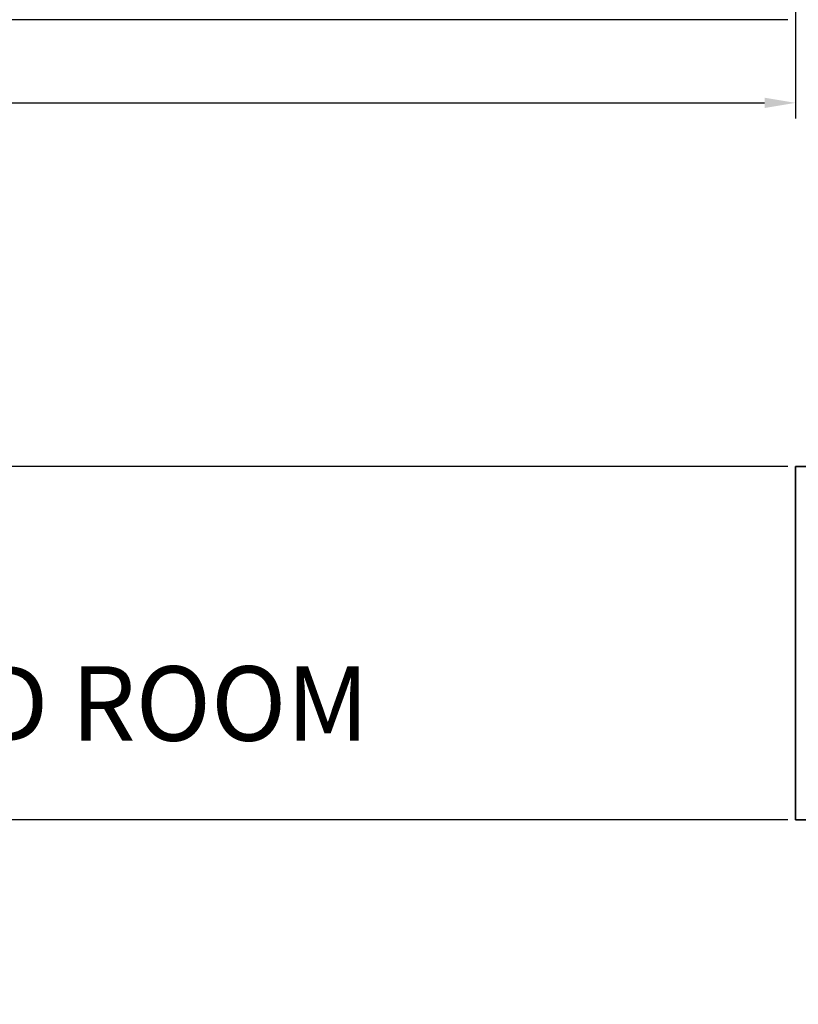
# Model space of a CAD drawing. Units: inches. Extents: x 2025 to 2528, y 1525 to 2336.
# Tile 14 of 18: x 2192 to 2255, y 2167 to 2246. Entities that reach past the tile are written whole.
import ezdxf

# ---------------------------------------------------------------- set-up
doc = ezdxf.new("R2010")
doc.units = ezdxf.units.IN
for name, color, linetype, lineweight in [('A-ANNO-DIMS', 2, 'Continuous', 18), ('A-AREA-IDEN', 7, 'Continuous', 25), ('A-FURN', 8, 'Continuous', 18), ('A-WALL', 7, 'Continuous', 35)]:
    doc.layers.add(name, color=color, linetype=linetype, lineweight=lineweight)
doc.styles.get("Standard").update_dxf_attribs({"font": 'arial.ttf'})
doc.dimstyles.new('Copy of ISO-25', dxfattribs={"dimtxt": 2.5, "dimasz": 2.5, "dimexe": 1.25, "dimexo": 0.625, "dimtad": 1, "dimdec": 1, "dimlunit": 4, "dimtxsty": 'Standard', "dimcen": 2.5, "dimadec": 0, "dimazin": 0, "dimtfac": 1, "dimtdec": 1, "dimtmove": 0, "dimatfit": 3, "dimfxl": 1, "dimarcsym": 0})

# ---------------------------------------------------------------- blocks, each defined once
blk = doc.blocks.new('*D6')
at = {"layer": 'A-ANNO-DIMS', "color": 0, "lineweight": -2, "transparency": 16777216}
for p, q in [((2075.013, 2282.787), (2075.013, 2237.927)), ((2255.013, 2282.787), (2255.013, 2237.927)), ((2077.513, 2239.177), (2252.513, 2239.177))]:
    blk.add_line(p, q, dxfattribs=at)
at = {"layer": 'A-ANNO-DIMS', "color": 0, "transparency": 16777216}
for points in [[(2077.513, 2239.594), (2077.513, 2238.761), (2075.013, 2239.177)], [(2252.513, 2239.594), (2252.513, 2238.761), (2255.013, 2239.177)]]:
    blk.add_solid(points, dxfattribs=at)
at = {"layer": 'Defpoints', "color": 0, "transparency": 16777216}
for p in [(2075.013, 2283.412), (2255.013, 2283.412), (2255.013, 2239.177)]:
    blk.add_point(p, dxfattribs=at)
at = {"layer": 'A-ANNO-DIMS', "color": 0, "transparency": 16777216, "insert": (2165.013, 2241.079), "char_height": 2.5, "attachment_point": 5}
blk.add_mtext("15'", dxfattribs=at)
blk = doc.blocks.new('A$C029D5C69')
for p, q in [((0.4164, 2.0693), (0.4164, 2.0066)), ((2.2315, 2.0693), (0.4164, 2.0693)), ((2.2315, 2.0066), (2.2315, 2.0693)), ((0, 1.606), (0, 2.0066)), ((0, 2.0066), (0.505, 2.0066)), ((0.0151, 1.6211), (0.0151, 1.9915)), ((0.0151, 1.9915), (0.4899, 1.9915)), ((0.4164, 2.0066), (2.2315, 2.0066)), ((0.4899, 1.9915), (0.4899, 1.6211)), ((0.505, 2.0066), (0.505, 1.606)), ((0.5252, 0.0351), (0.5252, 2.0066)), ((0.5403, 0.0502), (0.5403, 2.0066)), ((0.5706, 0.0805), (0.5706, 2.0066)), ((0.6869, 1.966), (0.6666, 2.0066)), ((0.7072, 2.0066), (0.6869, 1.966)), ((1.0902, 1.966), (1.0699, 2.0066)), ((1.1106, 2.0066), (1.0902, 1.966)), ((2.1114, 2.0087), (2.1114, 0.0351)), ((2.6479, 2.0066), (2.1429, 2.0066)), ((2.1429, 2.0066), (2.1429, 1.606)), ((2.6328, 1.9915), (2.158, 1.9915)), ((2.158, 1.9915), (2.158, 1.6211)), ((2.6328, 1.6211), (2.6328, 1.9915)), ((2.6479, 1.606), (2.6479, 2.0066)), ((0.6869, 1.9425), (0.6869, 1.966)), ((0.6869, 1.9425), (0.6869, 1.966)), ((1.0902, 1.9425), (1.0902, 1.966)), ((1.0902, 1.9425), (1.0902, 1.966)), ((1.8954, 1.9865), (1.3081, 1.9865)), ((1.8954, 1.9713), (1.3339, 1.9713)), ((1.3849, 1.9713), (1.3656, 1.952)), ((1.3945, 1.9713), (1.3714, 1.9483)), ((1.4249, 1.945), (1.3986, 1.9713)), ((1.4288, 1.9507), (1.4081, 1.9713)), ((1.487, 1.9713), (1.4664, 1.9507)), ((1.4966, 1.9713), (1.4703, 1.945)), ((1.527, 1.945), (1.5007, 1.9713)), ((1.5309, 1.9507), (1.5102, 1.9713)), ((1.5891, 1.9713), (1.5685, 1.9507)), ((1.5987, 1.9713), (1.5724, 1.945)), ((1.6291, 1.945), (1.6028, 1.9713)), ((1.633, 1.9507), (1.6123, 1.9713)), ((1.6912, 1.9713), (1.6706, 1.9507)), ((1.7008, 1.9713), (1.6745, 1.945)), ((1.7312, 1.945), (1.7049, 1.9713)), ((1.7351, 1.9507), (1.7144, 1.9713)), ((1.7933, 1.9713), (1.7727, 1.9507)), ((1.8029, 1.9713), (1.7766, 1.945)), ((1.8333, 1.945), (1.807, 1.9713)), ((1.8372, 1.9507), (1.8165, 1.9713)), ((1.8954, 1.9713), (1.8748, 1.9507)), ((1.9043, 1.9707), (1.8787, 1.945)), ((1.9354, 1.945), (1.9114, 1.969)), ((0.2689, 1.9609), (0.2689, 1.6764)), ((0.6634, 1.9425), (0.621, 1.9213)), ((0.6634, 1.9425), (0.621, 1.9213)), ((0.6869, 1.9425), (0.6634, 1.9425)), ((0.6869, 1.9425), (0.7104, 1.9425)), ((0.7528, 1.9213), (0.7104, 1.9425)), ((0.7528, 1.9213), (0.7104, 1.9425)), ((1.0668, 1.9425), (1.0244, 1.9213)), ((1.0668, 1.9425), (1.0244, 1.9213)), ((1.0902, 1.9425), (1.0668, 1.9425)), ((1.0902, 1.9425), (1.1137, 1.9425)), ((1.1561, 1.9213), (1.1137, 1.9425)), ((1.1561, 1.9213), (1.1137, 1.9425)), ((1.4249, 1.945), (1.4059, 1.926)), ((1.4288, 1.9394), (1.4116, 1.9222)), ((1.4476, 1.9507), (1.4288, 1.9507)), ((1.4288, 1.9393), (1.4476, 1.9393)), ((1.4476, 1.9507), (1.4664, 1.9507)), ((1.4664, 1.9393), (1.4476, 1.9393)), ((1.493, 1.9128), (1.4664, 1.9394)), ((1.4986, 1.9167), (1.4703, 1.945)), ((1.527, 1.945), (1.4986, 1.9167)), ((1.5309, 1.9394), (1.5043, 1.9128)), ((1.5497, 1.9507), (1.5309, 1.9507)), ((1.5309, 1.9393), (1.5497, 1.9393)), ((1.5497, 1.9507), (1.5685, 1.9507)), ((1.5685, 1.9393), (1.5497, 1.9393)), ((1.595, 1.9128), (1.5685, 1.9394)), ((1.6007, 1.9167), (1.5724, 1.945)), ((1.6291, 1.945), (1.6007, 1.9167)), ((1.633, 1.9394), (1.6064, 1.9128)), ((1.6518, 1.9507), (1.633, 1.9507)), ((1.633, 1.9393), (1.6518, 1.9393)), ((1.6518, 1.9507), (1.6706, 1.9507)), ((1.6706, 1.9393), (1.6518, 1.9393)), ((1.6971, 1.9128), (1.6706, 1.9394)), ((1.7028, 1.9167), (1.6745, 1.945)), ((1.7312, 1.945), (1.7028, 1.9167)), ((1.7351, 1.9394), (1.7085, 1.9128)), ((1.7539, 1.9507), (1.7351, 1.9507)), ((1.7351, 1.9393), (1.7539, 1.9393)), ((1.7539, 1.9507), (1.7727, 1.9507)), ((1.7727, 1.9393), (1.7539, 1.9393)), ((1.7992, 1.9128), (1.7727, 1.9394)), ((1.8049, 1.9167), (1.7766, 1.945)), ((1.8333, 1.945), (1.8049, 1.9167)), ((1.8372, 1.9394), (1.8106, 1.9128)), ((1.856, 1.9507), (1.8372, 1.9507)), ((1.8372, 1.9393), (1.856, 1.9393)), ((1.856, 1.9507), (1.8748, 1.9507)), ((1.8748, 1.9393), (1.856, 1.9393)), ((1.9013, 1.9128), (1.8748, 1.9394)), ((1.907, 1.9167), (1.8787, 1.945)), ((1.9354, 1.945), (1.907, 1.9167)), ((1.9393, 1.9394), (1.9127, 1.9128)), ((1.9393, 1.9393), (1.9404, 1.9393)), ((2.379, 1.9609), (2.379, 1.6764)), ((0.621, 1.9213), (0.5955, 1.8958)), ((0.7783, 1.8958), (0.7528, 1.9213)), ((1.0243, 1.9213), (0.9988, 1.8958)), ((1.1816, 1.8958), (1.1561, 1.9213)), ((1.9414, 1.688), (1.9414, 1.931)), ((1.9565, 1.688), (1.9565, 1.931)), ((0.5955, 1.8958), (0.5743, 1.8534)), ((0.7995, 1.8534), (0.7783, 1.8958)), ((0.9989, 1.8958), (0.9777, 1.8534)), ((1.2028, 1.8534), (1.1816, 1.8958)), ((1.493, 1.8752), (1.493, 1.9128)), ((1.5043, 1.8752), (1.5043, 1.9128)), ((1.595, 1.8752), (1.595, 1.9128)), ((1.6064, 1.8752), (1.6064, 1.9128)), ((1.6971, 1.8752), (1.6971, 1.9128)), ((1.7085, 1.8752), (1.7085, 1.9128)), ((1.7992, 1.8752), (1.7992, 1.9128)), ((1.8106, 1.8752), (1.8106, 1.9128)), ((1.9013, 1.8752), (1.9013, 1.9128)), ((1.9127, 1.8752), (1.9127, 1.9128)), ((1.493, 1.8752), (1.4867, 1.869)), ((1.4986, 1.8713), (1.4922, 1.8648)), ((1.527, 1.8429), (1.4986, 1.8713)), ((1.5309, 1.8486), (1.5043, 1.8752)), ((1.595, 1.8752), (1.5685, 1.8486)), ((1.6007, 1.8713), (1.5724, 1.8429)), ((1.6291, 1.8429), (1.6007, 1.8713)), ((1.633, 1.8486), (1.6064, 1.8752)), ((1.6971, 1.8752), (1.6706, 1.8486)), ((1.7028, 1.8713), (1.6745, 1.8429)), ((1.7312, 1.8429), (1.7028, 1.8713)), ((1.7351, 1.8486), (1.7085, 1.8752)), ((1.7992, 1.8752), (1.7727, 1.8486)), ((1.8049, 1.8713), (1.7766, 1.8429)), ((1.8333, 1.8429), (1.8049, 1.8713)), ((1.8372, 1.8486), (1.8106, 1.8752)), ((1.9013, 1.8752), (1.8748, 1.8486)), ((1.907, 1.8713), (1.8787, 1.8429)), ((1.9354, 1.8429), (1.907, 1.8713)), ((1.9393, 1.8486), (1.9127, 1.8752)), ((0.5743, 1.8534), (0.5706, 1.8515)), ((0.5743, 1.8534), (0.5706, 1.8515)), ((0.8419, 1.8322), (0.7995, 1.8534)), ((0.8419, 1.8322), (0.7995, 1.8534)), ((0.9777, 1.8534), (0.9353, 1.8322)), ((0.9777, 1.8534), (0.9353, 1.8322)), ((1.2452, 1.8322), (1.2028, 1.8534)), ((1.2452, 1.8322), (1.2028, 1.8534)), ((1.5497, 1.8486), (1.5309, 1.8486)), ((1.5497, 1.8486), (1.5685, 1.8486)), ((1.6518, 1.8486), (1.633, 1.8486)), ((1.6518, 1.8486), (1.6706, 1.8486)), ((1.7539, 1.8486), (1.7351, 1.8486)), ((1.7539, 1.8486), (1.7727, 1.8486)), ((1.856, 1.8486), (1.8372, 1.8486)), ((1.856, 1.8486), (1.8748, 1.8486)), ((1.9414, 1.8486), (1.9393, 1.8486)), ((0.8674, 1.8067), (0.8419, 1.8322)), ((0.9352, 1.8322), (0.9097, 1.8067)), ((1.2707, 1.8067), (1.2452, 1.8322)), ((1.527, 1.8429), (1.5242, 1.8401)), ((1.5309, 1.8373), (1.5295, 1.8359)), ((1.5309, 1.8373), (1.5497, 1.8373)), ((1.5685, 1.8373), (1.5497, 1.8373)), ((1.595, 1.8107), (1.5685, 1.8373)), ((1.6007, 1.8146), (1.5724, 1.8429)), ((1.6291, 1.8429), (1.6007, 1.8146)), ((1.633, 1.8373), (1.6064, 1.8107)), ((1.633, 1.8373), (1.6518, 1.8373)), ((1.6706, 1.8373), (1.6518, 1.8373)), ((1.6971, 1.8107), (1.6706, 1.8373)), ((1.7028, 1.8146), (1.6745, 1.8429)), ((1.7312, 1.8429), (1.7028, 1.8146)), ((1.7351, 1.8373), (1.7085, 1.8107)), ((1.7351, 1.8373), (1.7539, 1.8373)), ((1.7727, 1.8373), (1.7539, 1.8373)), ((1.7992, 1.8107), (1.7727, 1.8373)), ((1.8049, 1.8146), (1.7766, 1.8429)), ((1.8333, 1.8429), (1.8049, 1.8146)), ((1.8372, 1.8373), (1.8106, 1.8107)), ((1.8372, 1.8373), (1.856, 1.8373)), ((1.8748, 1.8373), (1.856, 1.8373)), ((1.9013, 1.8107), (1.8748, 1.8373)), ((1.907, 1.8146), (1.8787, 1.8429)), ((1.9354, 1.8429), (1.907, 1.8146)), ((1.9393, 1.8373), (1.9127, 1.8107)), ((1.9393, 1.8373), (1.9414, 1.8373)), ((0.1267, 1.8186), (0.4111, 1.8186)), ((0.8886, 1.7643), (0.8674, 1.8067)), ((0.9098, 1.8067), (0.8886, 1.7643)), ((1.2919, 1.7643), (1.2707, 1.8067)), ((1.595, 1.7806), (1.595, 1.8107)), ((1.6064, 1.7731), (1.6064, 1.8107)), ((1.6971, 1.7731), (1.6971, 1.8107)), ((1.7085, 1.7731), (1.7085, 1.8107)), ((1.7992, 1.7731), (1.7992, 1.8107)), ((1.8106, 1.7731), (1.8106, 1.8107)), ((1.9013, 1.7731), (1.9013, 1.8107)), ((1.9127, 1.7731), (1.9127, 1.8107)), ((2.2367, 1.8186), (2.5212, 1.8186)), ((1.2981, 1.7768), (1.2919, 1.7643)), ((1.633, 1.7465), (1.6064, 1.7731)), ((1.6971, 1.7731), (1.6706, 1.7465)), ((1.7351, 1.7465), (1.7085, 1.7731)), ((1.7992, 1.7731), (1.7727, 1.7465)), ((1.8372, 1.7465), (1.8106, 1.7731)), ((1.9013, 1.7731), (1.8748, 1.7465)), ((1.9393, 1.7465), (1.9127, 1.7731)), ((0.8886, 1.7408), (0.8886, 1.7643)), ((1.2919, 1.7519), (1.2919, 1.7643)), ((1.7028, 1.7692), (1.6745, 1.7408)), ((1.7312, 1.7408), (1.7028, 1.7692)), ((1.8049, 1.7692), (1.7766, 1.7408)), ((1.8333, 1.7408), (1.8049, 1.7692)), ((1.907, 1.7692), (1.8787, 1.7408)), ((1.9354, 1.7408), (1.907, 1.7692)), ((0.8651, 1.7408), (0.8227, 1.7196)), ((0.8651, 1.7408), (0.8227, 1.7196)), ((0.912, 1.7408), (0.8651, 1.7408)), ((0.9544, 1.7196), (0.912, 1.7408)), ((0.9544, 1.7196), (0.912, 1.7408)), ((1.2684, 1.7408), (1.226, 1.7196)), ((1.2684, 1.7408), (1.226, 1.7196)), ((1.2885, 1.7408), (1.2684, 1.7408)), ((1.6518, 1.7465), (1.633, 1.7465)), ((1.6443, 1.7352), (1.6518, 1.7352)), ((1.6518, 1.7465), (1.6706, 1.7465)), ((1.6706, 1.7352), (1.6518, 1.7352)), ((1.6971, 1.7086), (1.6706, 1.7352)), ((1.7028, 1.7125), (1.6745, 1.7408)), ((1.7312, 1.7408), (1.7028, 1.7125)), ((1.7351, 1.7352), (1.7085, 1.7086)), ((1.7539, 1.7465), (1.7351, 1.7465)), ((1.7351, 1.7352), (1.7539, 1.7352)), ((1.7539, 1.7465), (1.7727, 1.7465)), ((1.7727, 1.7352), (1.7539, 1.7352)), ((1.7992, 1.7086), (1.7727, 1.7352)), ((1.8049, 1.7125), (1.7766, 1.7408)), ((1.8333, 1.7408), (1.8049, 1.7125)), ((1.8372, 1.7352), (1.8106, 1.7086)), ((1.856, 1.7465), (1.8372, 1.7465)), ((1.8372, 1.7352), (1.856, 1.7352)), ((1.856, 1.7465), (1.8748, 1.7465)), ((1.8748, 1.7352), (1.856, 1.7352)), ((1.9013, 1.7086), (1.8748, 1.7352)), ((1.907, 1.7125), (1.8787, 1.7408)), ((1.9354, 1.7408), (1.907, 1.7125)), ((1.9393, 1.7352), (1.9127, 1.7086)), ((1.9414, 1.7465), (1.9393, 1.7465)), ((1.9393, 1.7352), (1.9414, 1.7352)), ((0.5766, 1.6941), (0.5706, 1.7002)), ((0.8227, 1.7196), (0.7972, 1.6941)), ((0.98, 1.6941), (0.9545, 1.7196)), ((1.226, 1.7196), (1.2005, 1.6941)), ((1.6971, 1.682), (1.6971, 1.7086)), ((1.7085, 1.671), (1.7085, 1.7086)), ((1.7992, 1.671), (1.7992, 1.7086)), ((1.8106, 1.671), (1.8106, 1.7086)), ((1.9013, 1.671), (1.9013, 1.7086)), ((1.9127, 1.671), (1.9127, 1.7086)), ((0.5978, 1.6517), (0.5766, 1.6941)), ((0.7972, 1.6941), (0.776, 1.6517)), ((1.0011, 1.6517), (0.9799, 1.6941)), ((1.2005, 1.6941), (1.1793, 1.6517)), ((2.5551, 1.6275), (2.5551, 1.696)), ((1.7318, 1.6477), (1.7085, 1.671)), ((1.7992, 1.671), (1.7759, 1.6477)), ((1.8049, 1.6671), (1.7855, 1.6477)), ((1.8244, 1.6477), (1.8049, 1.6671)), ((1.8339, 1.6477), (1.8106, 1.671)), ((1.9013, 1.671), (1.878, 1.6477)), ((1.907, 1.6671), (1.8876, 1.6477)), ((1.9202, 1.6539), (1.907, 1.6671)), ((1.926, 1.6577), (1.9127, 1.671)), ((0.6402, 1.6305), (0.5978, 1.6517)), ((0.6402, 1.6305), (0.5978, 1.6517)), ((0.6657, 1.605), (0.6402, 1.6305)), ((0.7336, 1.6305), (0.7081, 1.605)), ((0.776, 1.6517), (0.7336, 1.6305)), ((0.776, 1.6517), (0.7336, 1.6305)), ((1.0435, 1.6305), (1.0011, 1.6517)), ((1.0435, 1.6305), (1.0011, 1.6517)), ((1.0691, 1.605), (1.0436, 1.6305)), ((1.1369, 1.6305), (1.1114, 1.605)), ((1.1793, 1.6517), (1.1369, 1.6305)), ((1.1793, 1.6517), (1.1369, 1.6305)), ((1.8961, 1.6477), (1.7289, 1.6477)), ((1.8961, 1.6325), (1.7422, 1.6325)), ((0.505, 1.606), (0, 1.606)), ((0.4899, 1.6211), (0.0151, 1.6211)), ((0.6869, 1.5626), (0.6657, 1.605)), ((0.7081, 1.605), (0.6869, 1.5626)), ((1.0902, 1.5626), (1.069, 1.605)), ((1.1114, 1.605), (1.0902, 1.5626)), ((2.1429, 1.606), (2.6479, 1.606)), ((2.158, 1.6211), (2.6328, 1.6211)), ((0.6869, 1.5392), (0.6869, 1.5626)), ((0.6869, 1.5392), (0.6869, 1.5626)), ((1.0902, 1.5392), (1.0902, 1.5626)), ((1.0902, 1.5392), (1.0902, 1.5626)), ((0.6634, 1.5391), (0.621, 1.5179)), ((0.6634, 1.5391), (0.621, 1.5179)), ((0.6869, 1.5392), (0.6634, 1.5392)), ((0.6869, 1.5392), (0.7104, 1.5392)), ((0.7528, 1.5179), (0.7104, 1.5391)), ((0.7528, 1.5179), (0.7104, 1.5391)), ((1.0668, 1.5391), (1.0244, 1.5179)), ((1.0668, 1.5391), (1.0244, 1.5179)), ((1.0902, 1.5392), (1.0668, 1.5392)), ((1.0902, 1.5392), (1.1137, 1.5392)), ((1.1561, 1.5179), (1.1137, 1.5391)), ((1.1561, 1.5179), (1.1137, 1.5391)), ((0.621, 1.5179), (0.5955, 1.4924)), ((0.7783, 1.4924), (0.7528, 1.5179)), ((1.0243, 1.5179), (0.9988, 1.4924)), ((1.1816, 1.4924), (1.1561, 1.5179)), ((1.4277, 1.5179), (1.4022, 1.4924)), ((1.4534, 1.5308), (1.4277, 1.5179)), ((1.4534, 1.5308), (1.4277, 1.5179)), ((0.5955, 1.4925), (0.5743, 1.4501)), ((0.7995, 1.4501), (0.7783, 1.4925)), ((0.9989, 1.4925), (0.9777, 1.4501)), ((1.2028, 1.4501), (1.1816, 1.4925)), ((1.4022, 1.4925), (1.381, 1.4501)), ((1.6062, 1.4501), (1.5966, 1.4692)), ((0.5743, 1.45), (0.5706, 1.4481)), ((0.5743, 1.45), (0.5706, 1.4481)), ((0.8419, 1.4288), (0.7995, 1.45)), ((0.8419, 1.4288), (0.7995, 1.45)), ((0.9777, 1.45), (0.9353, 1.4288)), ((0.9777, 1.45), (0.9353, 1.4288)), ((1.2452, 1.4288), (1.2028, 1.45)), ((1.2452, 1.4288), (1.2028, 1.45)), ((1.381, 1.45), (1.3386, 1.4288)), ((1.381, 1.45), (1.3386, 1.4288)), ((1.6486, 1.4288), (1.6062, 1.45)), ((1.6486, 1.4288), (1.6062, 1.45)), ((0.8674, 1.4033), (0.8419, 1.4288)), ((0.9352, 1.4288), (0.9097, 1.4033)), ((1.2707, 1.4033), (1.2452, 1.4288)), ((1.3386, 1.4288), (1.3131, 1.4033)), ((1.6741, 1.4033), (1.6486, 1.4288)), ((0.5403, 1.4117), (0.5706, 1.4117)), ((0.8886, 1.361), (0.8674, 1.4034)), ((0.9098, 1.4034), (0.8886, 1.361)), ((1.2919, 1.361), (1.2707, 1.4034)), ((1.3131, 1.4034), (1.2919, 1.361)), ((1.6953, 1.361), (1.6741, 1.4034)), ((1.714, 1.3984), (1.6953, 1.361)), ((0.8886, 1.3375), (0.8886, 1.3609)), ((1.2919, 1.3375), (1.2919, 1.3609)), ((1.6953, 1.3375), (1.6953, 1.3609)), ((0.8651, 1.3374), (0.8227, 1.3162)), ((0.8651, 1.3374), (0.8227, 1.3162)), ((0.912, 1.3375), (0.8651, 1.3375)), ((0.9544, 1.3162), (0.912, 1.3374)), ((0.9544, 1.3162), (0.912, 1.3374)), ((1.2684, 1.3374), (1.226, 1.3162)), ((1.2684, 1.3374), (1.226, 1.3162)), ((1.3154, 1.3375), (1.2684, 1.3375)), ((1.3578, 1.3162), (1.3154, 1.3374)), ((1.3578, 1.3162), (1.3154, 1.3374)), ((1.6718, 1.3374), (1.6294, 1.3162)), ((1.6718, 1.3374), (1.6294, 1.3162)), ((1.7187, 1.3375), (1.6718, 1.3375)), ((1.7611, 1.3162), (1.7187, 1.3374)), ((1.7611, 1.3162), (1.7187, 1.3374)), ((0.5766, 1.2908), (0.5706, 1.2968)), ((0.8227, 1.3163), (0.7972, 1.2908)), ((0.98, 1.2908), (0.9545, 1.3163)), ((1.226, 1.3163), (1.2005, 1.2908)), ((1.3833, 1.2908), (1.3578, 1.3163)), ((1.6294, 1.3163), (1.6039, 1.2908)), ((1.7867, 1.2908), (1.7611, 1.3163)), ((0.5978, 1.2484), (0.5766, 1.2908)), ((0.7972, 1.2908), (0.776, 1.2484)), ((1.0011, 1.2484), (0.9799, 1.2908)), ((1.2005, 1.2908), (1.1793, 1.2484)), ((1.4045, 1.2484), (1.3833, 1.2908)), ((1.6039, 1.2908), (1.5827, 1.2484)), ((1.8078, 1.2484), (1.7866, 1.2908)), ((0.6402, 1.2271), (0.5978, 1.2483)), ((0.6402, 1.2271), (0.5978, 1.2483)), ((0.776, 1.2483), (0.7336, 1.2271)), ((0.776, 1.2483), (0.7336, 1.2271)), ((1.0435, 1.2271), (1.0011, 1.2483)), ((1.0435, 1.2271), (1.0011, 1.2483)), ((1.1793, 1.2483), (1.1369, 1.2271)), ((1.1793, 1.2483), (1.1369, 1.2271)), ((1.4469, 1.2271), (1.4045, 1.2483)), ((1.4469, 1.2271), (1.4045, 1.2483)), ((1.5827, 1.2483), (1.5403, 1.2271)), ((1.5827, 1.2483), (1.5403, 1.2271)), ((1.8502, 1.2271), (1.8078, 1.2483)), ((1.8502, 1.2271), (1.8078, 1.2483)), ((0.6657, 1.2017), (0.6402, 1.2272)), ((0.7336, 1.2272), (0.7081, 1.2017)), ((1.0691, 1.2017), (1.0436, 1.2272)), ((1.1369, 1.2272), (1.1114, 1.2017)), ((1.4724, 1.2017), (1.4469, 1.2272)), ((1.5403, 1.2272), (1.5148, 1.2017)), ((1.8758, 1.2017), (1.8503, 1.2272)), ((0.5403, 1.21), (0.5706, 1.21)), ((0.6869, 1.1593), (0.6657, 1.2017)), ((0.7081, 1.2017), (0.6869, 1.1593)), ((1.0902, 1.1593), (1.069, 1.2017)), ((1.1114, 1.2017), (1.0902, 1.1593)), ((1.4936, 1.1593), (1.4724, 1.2017)), ((1.5148, 1.2017), (1.4936, 1.1593)), ((1.8969, 1.1593), (1.8757, 1.2017)), ((1.9181, 1.2017), (1.8969, 1.1593)), ((1.9215, 1.2051), (1.9181, 1.2017)), ((0.6869, 1.1358), (0.6869, 1.1593)), ((0.6869, 1.1358), (0.6869, 1.1593)), ((1.0902, 1.1358), (1.0902, 1.1593)), ((1.0902, 1.1358), (1.0902, 1.1593)), ((1.4936, 1.1358), (1.4936, 1.1593)), ((1.4936, 1.1358), (1.4936, 1.1593)), ((1.8969, 1.1358), (1.8969, 1.1593)), ((1.8969, 1.1358), (1.8969, 1.1593)), ((0.6634, 1.1358), (0.621, 1.1146)), ((0.6634, 1.1358), (0.621, 1.1146)), ((0.6869, 1.1358), (0.6634, 1.1358)), ((0.6869, 1.1358), (0.7104, 1.1358)), ((0.7528, 1.1146), (0.7104, 1.1358)), ((0.7528, 1.1146), (0.7104, 1.1358)), ((1.0668, 1.1358), (1.0244, 1.1146)), ((1.0668, 1.1358), (1.0244, 1.1146)), ((1.0902, 1.1358), (1.0668, 1.1358)), ((1.0902, 1.1358), (1.1137, 1.1358)), ((1.1561, 1.1146), (1.1137, 1.1358)), ((1.1561, 1.1146), (1.1137, 1.1358)), ((1.4701, 1.1358), (1.4277, 1.1146)), ((1.4701, 1.1358), (1.4277, 1.1146)), ((1.4936, 1.1358), (1.4701, 1.1358)), ((1.4936, 1.1358), (1.5171, 1.1358)), ((1.5595, 1.1146), (1.5171, 1.1358)), ((1.5595, 1.1146), (1.5171, 1.1358)), ((1.8735, 1.1358), (1.8311, 1.1146)), ((1.8735, 1.1358), (1.8311, 1.1146)), ((1.8969, 1.1358), (1.8735, 1.1358)), ((1.8969, 1.1358), (1.9204, 1.1358)), ((1.9628, 1.1146), (1.9204, 1.1358)), ((1.9628, 1.1146), (1.9204, 1.1358)), ((0.621, 1.1146), (0.5955, 1.0891)), ((0.7783, 1.0891), (0.7528, 1.1146)), ((1.0243, 1.1146), (0.9988, 1.0891)), ((1.1816, 1.0891), (1.1561, 1.1146)), ((1.4277, 1.1146), (1.4022, 1.0891)), ((1.585, 1.0891), (1.5595, 1.1146)), ((1.831, 1.1146), (1.8055, 1.0891)), ((1.9883, 1.0891), (1.9628, 1.1146)), ((0.5955, 1.0891), (0.5743, 1.0467)), ((0.7995, 1.0467), (0.7783, 1.0891)), ((0.9989, 1.0891), (0.9777, 1.0467)), ((1.2028, 1.0467), (1.1816, 1.0891)), ((1.4022, 1.0891), (1.381, 1.0467)), ((1.6062, 1.0467), (1.585, 1.0891)), ((1.8056, 1.0891), (1.7844, 1.0467)), ((2.0095, 1.0467), (1.9883, 1.0891)), ((0.5743, 1.0467), (0.5706, 1.0448)), ((0.5743, 1.0467), (0.5706, 1.0448)), ((0.8419, 1.0255), (0.7995, 1.0467)), ((0.8419, 1.0255), (0.7995, 1.0467)), ((0.9777, 1.0467), (0.9353, 1.0255)), ((0.9777, 1.0467), (0.9353, 1.0255)), ((1.2452, 1.0255), (1.2028, 1.0467)), ((1.2452, 1.0255), (1.2028, 1.0467)), ((1.381, 1.0467), (1.3386, 1.0255)), ((1.381, 1.0467), (1.3386, 1.0255)), ((1.6486, 1.0255), (1.6062, 1.0467)), ((1.6486, 1.0255), (1.6062, 1.0467)), ((1.7844, 1.0467), (1.742, 1.0255)), ((1.7844, 1.0467), (1.742, 1.0255)), ((2.0276, 1.0376), (2.0095, 1.0467)), ((2.0276, 1.0376), (2.0095, 1.0467)), ((0.8674, 1), (0.8419, 1.0255)), ((0.9352, 1.0255), (0.9097, 1)), ((1.2707, 1), (1.2452, 1.0255)), ((1.3386, 1.0255), (1.3131, 1)), ((1.6741, 1), (1.6486, 1.0255)), ((1.7419, 1.0255), (1.7164, 1)), ((0.8886, 0.9576), (0.8674, 1)), ((0.9098, 1), (0.8886, 0.9576)), ((1.2919, 0.9576), (1.2707, 1)), ((1.3131, 1), (1.2919, 0.9576)), ((1.6953, 0.9576), (1.6741, 1)), ((1.7165, 1), (1.6953, 0.9576)), ((0.8651, 0.9341), (0.8227, 0.9129)), ((0.8651, 0.9341), (0.8227, 0.9129)), ((0.912, 0.9341), (0.8651, 0.9341)), ((0.8886, 0.9341), (0.8886, 0.9576)), ((0.9544, 0.9129), (0.912, 0.9341)), ((0.9544, 0.9129), (0.912, 0.9341)), ((1.2684, 0.9341), (1.226, 0.9129)), ((1.2684, 0.9341), (1.226, 0.9129)), ((1.3154, 0.9341), (1.2684, 0.9341)), ((1.2919, 0.9341), (1.2919, 0.9576)), ((1.3578, 0.9129), (1.3154, 0.9341)), ((1.3578, 0.9129), (1.3154, 0.9341)), ((1.6718, 0.9341), (1.6294, 0.9129)), ((1.6718, 0.9341), (1.6294, 0.9129)), ((1.7187, 0.9341), (1.6718, 0.9341)), ((1.6953, 0.9341), (1.6953, 0.9576)), ((1.7611, 0.9129), (1.7187, 0.9341)), ((1.7611, 0.9129), (1.7187, 0.9341)), ((2.066, 0.9457), (2.066, 0.0805)), ((0.8227, 0.9129), (0.7972, 0.8874)), ((0.98, 0.8874), (0.9545, 0.9129)), ((1.226, 0.9129), (1.2005, 0.8874)), ((1.3833, 0.8874), (1.3578, 0.9129)), ((1.6294, 0.9129), (1.6039, 0.8874)), ((1.7867, 0.8874), (1.7611, 0.9129)), ((2.0327, 0.9129), (2.0072, 0.8874)), ((2.066, 0.9295), (2.0327, 0.9129)), ((2.066, 0.9295), (2.0327, 0.9129)), ((0.5766, 0.8874), (0.5706, 0.8935)), ((0.5978, 0.845), (0.5766, 0.8874)), ((0.7972, 0.8874), (0.776, 0.845)), ((1.0011, 0.845), (0.9799, 0.8874)), ((1.2005, 0.8874), (1.1793, 0.845)), ((1.4045, 0.845), (1.3833, 0.8874)), ((1.6039, 0.8874), (1.5827, 0.845)), ((1.8078, 0.845), (1.7866, 0.8874)), ((2.0072, 0.8874), (1.986, 0.845)), ((0.6402, 0.8238), (0.5978, 0.845)), ((0.6402, 0.8238), (0.5978, 0.845)), ((0.776, 0.845), (0.7336, 0.8238)), ((0.776, 0.845), (0.7336, 0.8238)), ((1.0435, 0.8238), (1.0011, 0.845)), ((1.0435, 0.8238), (1.0011, 0.845)), ((1.1793, 0.845), (1.1369, 0.8238)), ((1.1793, 0.845), (1.1369, 0.8238)), ((1.4469, 0.8238), (1.4045, 0.845)), ((1.4469, 0.8238), (1.4045, 0.845)), ((1.5827, 0.845), (1.5403, 0.8238)), ((1.5827, 0.845), (1.5403, 0.8238)), ((1.8502, 0.8238), (1.8078, 0.845)), ((1.8502, 0.8238), (1.8078, 0.845)), ((1.986, 0.845), (1.9436, 0.8238)), ((1.986, 0.845), (1.9436, 0.8238)), ((0.6657, 0.7983), (0.6402, 0.8238)), ((0.7336, 0.8238), (0.7081, 0.7983)), ((1.0691, 0.7983), (1.0436, 0.8238)), ((1.1369, 0.8238), (1.1114, 0.7983)), ((1.4724, 0.7983), (1.4469, 0.8238)), ((1.5403, 0.8238), (1.5148, 0.7983)), ((1.8758, 0.7983), (1.8503, 0.8238)), ((1.9436, 0.8238), (1.9181, 0.7983)), ((2.0962, 0.8369), (2.0962, 0.0502)), ((0.6869, 0.7559), (0.6657, 0.7983)), ((0.7081, 0.7983), (0.6869, 0.7559)), ((1.0902, 0.7559), (1.069, 0.7983)), ((1.1114, 0.7983), (1.0902, 0.7559)), ((1.4936, 0.7559), (1.4724, 0.7983)), ((1.5148, 0.7983), (1.4936, 0.7559)), ((1.8969, 0.7559), (1.8757, 0.7983)), ((1.9181, 0.7983), (1.8969, 0.7559)), ((0.6869, 0.7325), (0.6869, 0.7559)), ((0.6869, 0.7325), (0.6869, 0.7559)), ((1.0902, 0.7325), (1.0902, 0.7559)), ((1.0902, 0.7325), (1.0902, 0.7559)), ((1.2024, 0.7028), (1.2503, 0.7507)), ((1.4936, 0.7325), (1.4936, 0.7559)), ((1.4936, 0.7325), (1.4936, 0.7559)), ((1.8969, 0.7325), (1.8969, 0.7559)), ((1.8969, 0.7325), (1.8969, 0.7559)), ((0.6634, 0.7324), (0.621, 0.7112)), ((0.6634, 0.7324), (0.621, 0.7112)), ((0.6869, 0.7325), (0.6634, 0.7325)), ((0.6869, 0.7325), (0.7104, 0.7325)), ((0.7528, 0.7112), (0.7104, 0.7324)), ((0.7528, 0.7112), (0.7104, 0.7324)), ((1.0668, 0.7324), (1.0244, 0.7112)), ((1.0668, 0.7324), (1.0244, 0.7112)), ((1.0902, 0.7325), (1.0668, 0.7325)), ((1.0902, 0.7325), (1.1137, 0.7325)), ((1.1561, 0.7112), (1.1137, 0.7324)), ((1.1561, 0.7112), (1.1137, 0.7324)), ((1.4701, 0.7324), (1.4277, 0.7112)), ((1.4701, 0.7324), (1.4277, 0.7112)), ((1.4936, 0.7325), (1.4701, 0.7325)), ((1.4936, 0.7325), (1.5171, 0.7325)), ((1.5595, 0.7112), (1.5171, 0.7324)), ((1.5595, 0.7112), (1.5171, 0.7324)), ((1.8735, 0.7324), (1.8311, 0.7112)), ((1.8735, 0.7324), (1.8311, 0.7112)), ((1.8969, 0.7325), (1.8735, 0.7325)), ((1.8969, 0.7325), (1.9204, 0.7325)), ((1.9628, 0.7112), (1.9204, 0.7324)), ((1.9628, 0.7112), (1.9204, 0.7324)), ((0.621, 0.7113), (0.5955, 0.6858)), ((0.7783, 0.6858), (0.7528, 0.7113)), ((1.0243, 0.7113), (0.9988, 0.6858)), ((1.1816, 0.6858), (1.1561, 0.7113)), ((1.4277, 0.7113), (1.4022, 0.6858)), ((1.585, 0.6858), (1.5595, 0.7113)), ((1.831, 0.7113), (1.8055, 0.6858)), ((1.9883, 0.6858), (1.9628, 0.7113)), ((0.5955, 0.6858), (0.5743, 0.6434)), ((0.7995, 0.6434), (0.7783, 0.6858)), ((0.9989, 0.6858), (0.9777, 0.6434)), ((1.2028, 0.6434), (1.1816, 0.6858)), ((1.4022, 0.6858), (1.381, 0.6434)), ((1.6062, 0.6434), (1.585, 0.6858)), ((1.8056, 0.6858), (1.7844, 0.6434)), ((2.0095, 0.6434), (1.9883, 0.6858)), ((0.5743, 0.6433), (0.5706, 0.6414)), ((0.5743, 0.6433), (0.5706, 0.6414)), ((0.8419, 0.6221), (0.7995, 0.6433)), ((0.8419, 0.6221), (0.7995, 0.6433)), ((0.9777, 0.6433), (0.9353, 0.6221)), ((0.9777, 0.6433), (0.9353, 0.6221)), ((1.2452, 0.6221), (1.2028, 0.6433)), ((1.2452, 0.6221), (1.2028, 0.6433)), ((1.381, 0.6433), (1.3386, 0.6221)), ((1.381, 0.6433), (1.3386, 0.6221)), ((1.6486, 0.6221), (1.6062, 0.6433)), ((1.6486, 0.6221), (1.6062, 0.6433)), ((1.7844, 0.6433), (1.742, 0.6221)), ((1.7844, 0.6433), (1.742, 0.6221)), ((2.0519, 0.6221), (2.0095, 0.6433)), ((2.0519, 0.6221), (2.0095, 0.6433)), ((0.8674, 0.5967), (0.8419, 0.6222)), ((0.9352, 0.6222), (0.9097, 0.5967)), ((1.2707, 0.5967), (1.2452, 0.6222)), ((1.3386, 0.6222), (1.3131, 0.5967)), ((1.6741, 0.5967), (1.6486, 0.6222)), ((1.7419, 0.6222), (1.7164, 0.5967)), ((2.066, 0.6081), (2.0519, 0.6222)), ((0.8886, 0.5543), (0.8674, 0.5967)), ((0.9098, 0.5967), (0.8886, 0.5543)), ((1.2919, 0.5543), (1.2707, 0.5967)), ((1.3131, 0.5967), (1.2919, 0.5543)), ((1.6953, 0.5543), (1.6741, 0.5967)), ((1.7165, 0.5967), (1.6953, 0.5543)), ((0.8886, 0.5308), (0.8886, 0.5543)), ((1.2919, 0.5308), (1.2919, 0.5543)), ((1.6953, 0.5308), (1.6953, 0.5543)), ((0.8651, 0.5308), (0.8227, 0.5096)), ((0.8651, 0.5308), (0.8227, 0.5096)), ((0.912, 0.5308), (0.8651, 0.5308)), ((0.9544, 0.5096), (0.912, 0.5308)), ((0.9544, 0.5096), (0.912, 0.5308)), ((1.2684, 0.5308), (1.226, 0.5096)), ((1.2684, 0.5308), (1.226, 0.5096)), ((1.3154, 0.5308), (1.2684, 0.5308)), ((1.3578, 0.5096), (1.3154, 0.5308)), ((1.3578, 0.5096), (1.3154, 0.5308)), ((1.6718, 0.5308), (1.6294, 0.5096)), ((1.6718, 0.5308), (1.6294, 0.5096)), ((1.7187, 0.5308), (1.6718, 0.5308)), ((1.7611, 0.5096), (1.7187, 0.5308)), ((1.7611, 0.5096), (1.7187, 0.5308)), ((0.8227, 0.5096), (0.7972, 0.4841)), ((0.98, 0.4841), (0.9545, 0.5096)), ((1.226, 0.5096), (1.2005, 0.4841)), ((1.3833, 0.4841), (1.3578, 0.5096)), ((1.6294, 0.5096), (1.6039, 0.4841)), ((1.7867, 0.4841), (1.7611, 0.5096)), ((2.0327, 0.5096), (2.0072, 0.4841)), ((2.066, 0.5262), (2.0327, 0.5096)), ((2.066, 0.5262), (2.0327, 0.5096)), ((0.5766, 0.4841), (0.5706, 0.4901)), ((0.5978, 0.4417), (0.5766, 0.4841)), ((0.7972, 0.4841), (0.776, 0.4417)), ((1.0011, 0.4417), (0.9799, 0.4841)), ((1.2005, 0.4841), (1.1793, 0.4417)), ((1.4045, 0.4417), (1.3833, 0.4841)), ((1.6039, 0.4841), (1.5827, 0.4417)), ((1.8078, 0.4417), (1.7866, 0.4841)), ((2.0072, 0.4841), (1.986, 0.4417)), ((0.6402, 0.4205), (0.5978, 0.4417)), ((0.6402, 0.4205), (0.5978, 0.4417)), ((0.776, 0.4417), (0.7336, 0.4205)), ((0.776, 0.4417), (0.7336, 0.4205)), ((1.0435, 0.4205), (1.0011, 0.4417)), ((1.0435, 0.4205), (1.0011, 0.4417)), ((1.1793, 0.4417), (1.1369, 0.4205)), ((1.1793, 0.4417), (1.1369, 0.4205)), ((1.4469, 0.4205), (1.4045, 0.4417)), ((1.4469, 0.4205), (1.4045, 0.4417)), ((1.5827, 0.4417), (1.5403, 0.4205)), ((1.5827, 0.4417), (1.5403, 0.4205)), ((1.8502, 0.4205), (1.8078, 0.4417)), ((1.8502, 0.4205), (1.8078, 0.4417)), ((1.986, 0.4417), (1.9436, 0.4205)), ((1.986, 0.4417), (1.9436, 0.4205)), ((0.6657, 0.395), (0.6402, 0.4205)), ((0.7336, 0.4205), (0.7081, 0.395)), ((1.0691, 0.395), (1.0436, 0.4205)), ((1.1369, 0.4205), (1.1114, 0.395)), ((1.4724, 0.395), (1.4469, 0.4205)), ((1.5403, 0.4205), (1.5148, 0.395)), ((1.8758, 0.395), (1.8503, 0.4205)), ((1.9436, 0.4205), (1.9181, 0.395)), ((0.6869, 0.3526), (0.6657, 0.395)), ((0.7081, 0.395), (0.6869, 0.3526)), ((1.0902, 0.3526), (1.069, 0.395)), ((1.1114, 0.395), (1.0902, 0.3526)), ((1.4936, 0.3526), (1.4724, 0.395)), ((1.5148, 0.395), (1.4936, 0.3526)), ((1.8969, 0.3526), (1.8757, 0.395)), ((1.9181, 0.395), (1.8969, 0.3526)), ((0.6869, 0.3291), (0.6869, 0.3526)), ((0.6869, 0.3291), (0.6869, 0.3526)), ((1.0902, 0.3291), (1.0902, 0.3526)), ((1.0902, 0.3291), (1.0902, 0.3526)), ((1.4936, 0.3291), (1.4936, 0.3526)), ((1.4936, 0.3291), (1.4936, 0.3526)), ((1.8969, 0.3291), (1.8969, 0.3526)), ((1.8969, 0.3291), (1.8969, 0.3526)), ((0.6634, 0.3291), (0.621, 0.3079)), ((0.6634, 0.3291), (0.621, 0.3079)), ((0.6869, 0.3291), (0.6634, 0.3291)), ((0.6869, 0.3291), (0.7104, 0.3291)), ((0.7528, 0.3079), (0.7104, 0.3291)), ((0.7528, 0.3079), (0.7104, 0.3291)), ((1.0668, 0.3291), (1.0244, 0.3079)), ((1.0668, 0.3291), (1.0244, 0.3079)), ((1.0902, 0.3291), (1.0668, 0.3291)), ((1.0902, 0.3291), (1.1137, 0.3291)), ((1.1561, 0.3079), (1.1137, 0.3291)), ((1.1561, 0.3079), (1.1137, 0.3291)), ((1.4701, 0.3291), (1.4277, 0.3079)), ((1.4701, 0.3291), (1.4277, 0.3079)), ((1.4936, 0.3291), (1.4701, 0.3291)), ((1.4936, 0.3291), (1.5171, 0.3291)), ((1.5595, 0.3079), (1.5171, 0.3291)), ((1.5595, 0.3079), (1.5171, 0.3291)), ((1.8735, 0.3291), (1.8311, 0.3079)), ((1.8735, 0.3291), (1.8311, 0.3079)), ((1.8969, 0.3291), (1.8735, 0.3291)), ((1.8969, 0.3291), (1.9204, 0.3291)), ((1.9628, 0.3079), (1.9204, 0.3291)), ((1.9628, 0.3079), (1.9204, 0.3291)), ((0.621, 0.3079), (0.5955, 0.2824)), ((0.7783, 0.2824), (0.7528, 0.3079)), ((1.0243, 0.3079), (0.9988, 0.2824)), ((1.1816, 0.2824), (1.1561, 0.3079)), ((1.4277, 0.3079), (1.4022, 0.2824)), ((1.585, 0.2824), (1.5595, 0.3079)), ((1.831, 0.3079), (1.8055, 0.2824)), ((1.9883, 0.2824), (1.9628, 0.3079)), ((0.5955, 0.2824), (0.5743, 0.24)), ((0.7995, 0.24), (0.7783, 0.2824)), ((0.9989, 0.2824), (0.9777, 0.24)), ((1.2028, 0.24), (1.1816, 0.2824)), ((1.4022, 0.2824), (1.381, 0.24)), ((1.6062, 0.24), (1.585, 0.2824)), ((1.8056, 0.2824), (1.7844, 0.24)), ((2.0095, 0.24), (1.9883, 0.2824)), ((0.5743, 0.24), (0.5706, 0.2381)), ((0.5743, 0.24), (0.5706, 0.2381)), ((0.8419, 0.2188), (0.7995, 0.24)), ((0.8419, 0.2188), (0.7995, 0.24)), ((0.9777, 0.24), (0.9353, 0.2188)), ((0.9777, 0.24), (0.9353, 0.2188)), ((1.2452, 0.2188), (1.2028, 0.24)), ((1.2452, 0.2188), (1.2028, 0.24)), ((1.381, 0.24), (1.3386, 0.2188)), ((1.381, 0.24), (1.3386, 0.2188)), ((1.6486, 0.2188), (1.6062, 0.24)), ((1.6486, 0.2188), (1.6062, 0.24)), ((1.7844, 0.24), (1.742, 0.2188)), ((1.7844, 0.24), (1.742, 0.2188)), ((2.0519, 0.2188), (2.0095, 0.24)), ((2.0519, 0.2188), (2.0095, 0.24)), ((0.8674, 0.1933), (0.8419, 0.2188)), ((0.9352, 0.2188), (0.9097, 0.1933)), ((1.2707, 0.1933), (1.2452, 0.2188)), ((1.3386, 0.2188), (1.3131, 0.1933)), ((1.6741, 0.1933), (1.6486, 0.2188)), ((1.7419, 0.2188), (1.7164, 0.1933)), ((2.066, 0.2047), (2.0519, 0.2188)), ((0.8886, 0.1509), (0.8674, 0.1933)), ((0.9098, 0.1933), (0.8886, 0.1509)), ((1.2919, 0.1509), (1.2707, 0.1933)), ((1.3131, 0.1933), (1.2919, 0.1509)), ((1.6953, 0.1509), (1.6741, 0.1933)), ((1.7165, 0.1933), (1.6953, 0.1509)), ((0.8886, 0.1275), (0.8886, 0.1509)), ((1.2919, 0.1275), (1.2919, 0.1509)), ((1.6953, 0.1275), (1.6953, 0.1509)), ((0.8651, 0.1274), (0.8227, 0.1062)), ((0.8651, 0.1274), (0.8227, 0.1062)), ((0.912, 0.1275), (0.8651, 0.1275)), ((0.9544, 0.1062), (0.912, 0.1274)), ((0.9544, 0.1062), (0.912, 0.1274)), ((1.2684, 0.1274), (1.226, 0.1062)), ((1.2684, 0.1274), (1.226, 0.1062)), ((1.3154, 0.1275), (1.2684, 0.1275)), ((1.3578, 0.1062), (1.3154, 0.1274)), ((1.3578, 0.1062), (1.3154, 0.1274)), ((1.6718, 0.1274), (1.6294, 0.1062)), ((1.6718, 0.1274), (1.6294, 0.1062)), ((1.7187, 0.1275), (1.6718, 0.1275)), ((1.7611, 0.1062), (1.7187, 0.1274)), ((1.7611, 0.1062), (1.7187, 0.1274)), ((2.066, 0.1228), (2.0327, 0.1062)), ((2.066, 0.1228), (2.0327, 0.1062)), ((0.8227, 0.1062), (0.7972, 0.0807)), ((0.98, 0.0807), (0.9545, 0.1062)), ((1.226, 0.1062), (1.2005, 0.0807)), ((1.3833, 0.0807), (1.3578, 0.1062)), ((1.6294, 0.1062), (1.6039, 0.0807)), ((1.7867, 0.0807), (1.7611, 0.1062)), ((2.0327, 0.1062), (2.0072, 0.0807)), ((0.5766, 0.0807), (0.5706, 0.0868)), ((0.5978, 0.0384), (0.5766, 0.0808)), ((0.7972, 0.0808), (0.776, 0.0384)), ((1.0011, 0.0384), (0.9799, 0.0808)), ((1.2005, 0.0808), (1.1793, 0.0384)), ((1.4045, 0.0384), (1.3833, 0.0808)), ((1.6039, 0.0808), (1.5827, 0.0384)), ((1.8078, 0.0384), (1.7866, 0.0808)), ((2.0072, 0.0808), (1.986, 0.0384)), ((0.6402, 0.0171), (0.5978, 0.0383)), ((0.6402, 0.0171), (0.5978, 0.0383)), ((2.0309, 0.0454), (0.6056, 0.0454)), ((0.776, 0.0383), (0.7336, 0.0171)), ((0.776, 0.0383), (0.7336, 0.0171)), ((1.0435, 0.0171), (1.0011, 0.0383)), ((1.0435, 0.0171), (1.0011, 0.0383)), ((1.1793, 0.0383), (1.1369, 0.0171)), ((1.1793, 0.0383), (1.1369, 0.0171)), ((1.4469, 0.0171), (1.4045, 0.0383)), ((1.4469, 0.0171), (1.4045, 0.0383)), ((1.5827, 0.0383), (1.5403, 0.0171)), ((1.5827, 0.0383), (1.5403, 0.0171)), ((1.8502, 0.0171), (1.8078, 0.0383)), ((1.8502, 0.0171), (1.8078, 0.0383)), ((1.986, 0.0383), (1.9436, 0.0171)), ((1.986, 0.0383), (1.9436, 0.0171)), ((2.0763, 0), (0.5603, 0)), ((2.0612, 0.0151), (0.5754, 0.0151)), ((0.6523, 0.005), (0.6402, 0.0171)), ((0.7336, 0.0171), (0.7215, 0.005)), ((1.0557, 0.005), (1.0436, 0.0171)), ((1.1369, 0.0171), (1.1248, 0.005)), ((1.459, 0.005), (1.4469, 0.0171)), ((1.5403, 0.0171), (1.5282, 0.005)), ((1.8623, 0.005), (1.8503, 0.0171)), ((1.9436, 0.0171), (1.9315, 0.005))]:
    blk.add_line(p, q)
at = {"ltscale": 0.005}
for p, q in [((0.4899, 1.6568), (0.0151, 1.9915)), ((0.0151, 1.6568), (0.4899, 1.9915)), ((2.6328, 1.6568), (2.158, 1.9915)), ((2.158, 1.6568), (2.6328, 1.9915)), ((0.0151, 1.6568), (0.4899, 1.6568)), ((2.6328, 1.6568), (2.158, 1.6568))]:
    blk.add_line(p, q, dxfattribs=at)
for centre, radius in [((0.2689, 1.8186), 0.1191), ((2.379, 1.8186), 0.1191), ((0.2689, 1.8186), 0.0711), ((2.379, 1.8186), 0.0711)]:
    blk.add_circle(centre, radius)
for centre, radius, start, end in [((0.2843, 0.0157), 0.6251, 10.2961, 13.2684), ((0.6056, 0.0805), 0.0351, 180, 270), ((2.0309, 0.0805), 0.0351, 270, 0), ((0.5754, 0.0502), 0.0351, 180, 270), ((2.0612, 0.0502), 0.0351, 270, 0), ((0.5603, 0.0351), 0.0351, 180, 270), ((2.0763, 0.0351), 0.0351, 270, 0)]:
    blk.add_arc(centre, radius, start, end)
for centre, major_axis, ratio, start_param, end_param in [((0.8506, 1.8527), (-0.4556, 0), 0.89, 2.430919, 3.53111), ((0.3667, 0.6698), (1.7398, 0.1668), 0.88072, -0.045073, 0.941433), ((1.8961, 1.931), (-0.0453, 0), 0.89, 3.141593, 4.712389), ((1.8961, 1.688), (-0.0453, 0), 0.89, 1.570796, 3.141593), ((1.0874, 0.6748), (1.021, 0.1213), 0.889348, -0.031673, 1.359628)]:
    blk.add_ellipse(centre, major_axis=major_axis, ratio=ratio, start_param=start_param, end_param=end_param)
for points, knots in [([(1.9565, 1.931), (1.9565, 1.9336), (1.9563, 1.9362), (1.9553, 1.9428), (1.9543, 1.9467), (1.9512, 1.9541), (1.9493, 1.9577), (1.9446, 1.9643), (1.942, 1.9674), (1.936, 1.9729), (1.9327, 1.9753), (1.9257, 1.9795), (1.922, 1.9813), (1.9142, 1.9841), (1.9102, 1.9851), (1.9028, 1.9862), (1.8995, 1.9865), (1.8961, 1.9865)], [3.141593, 3.141593, 3.141593, 3.141593, 3.277614, 3.277614, 3.488082, 3.488082, 3.698551, 3.698551, 3.909019, 3.909019, 4.119488, 4.119488, 4.329956, 4.329956, 4.540424, 4.540424, 4.712389, 4.712389, 4.712389, 4.712389]), ([(1.8961, 1.6325), (1.899, 1.6325), (1.9019, 1.6327), (1.9101, 1.6338), (1.9153, 1.6352), (1.9253, 1.6392), (1.93, 1.6418), (1.9385, 1.6481), (1.9423, 1.6519), (1.9481, 1.6594), (1.9503, 1.663), (1.9537, 1.6707), (1.955, 1.6747), (1.9563, 1.6818), (1.9565, 1.6849), (1.9565, 1.688)], [1.570796, 1.570796, 1.570796, 1.570796, 1.718836, 1.718836, 1.993452, 1.993452, 2.268068, 2.268068, 2.542684, 2.542684, 2.761386, 2.761386, 2.980087, 2.980087, 3.141593, 3.141593, 3.141593, 3.141593])]:
    blk.add_open_spline(points, degree=3, knots=knots)
blk = doc.blocks.new('*D77')
at = {"layer": 'A-ANNO-DIMS', "color": 0, "lineweight": -2, "transparency": 16777216}
for p, q in [((2254.388, 2181.412), (2027.213, 2181.412)), ((2028.463, 2153.912), (2028.463, 2178.912)), ((2254.388, 2151.412), (2027.213, 2151.412))]:
    blk.add_line(p, q, dxfattribs=at)
at = {"layer": 'A-ANNO-DIMS', "color": 0, "transparency": 16777216}
for points in [[(2028.046, 2178.912), (2028.88, 2178.912), (2028.463, 2181.412)], [(2028.046, 2153.912), (2028.88, 2153.912), (2028.463, 2151.412)]]:
    blk.add_solid(points, dxfattribs=at)
at = {"layer": 'Defpoints', "color": 0, "transparency": 16777216}
for p in [(2028.463, 2181.412), (2255.013, 2181.412), (2255.013, 2151.412)]:
    blk.add_point(p, dxfattribs=at)
at = {"layer": 'A-ANNO-DIMS', "color": 0, "transparency": 16777216, "insert": (2026.561, 2166.412), "char_height": 2.5, "attachment_point": 5, "rotation": 90}
blk.add_mtext('2\'-6"', dxfattribs=at)
blk = doc.blocks.new('*D78')
at = {"layer": 'A-ANNO-DIMS', "color": 0, "lineweight": -2, "transparency": 16777216}
for p, q in [((2254.388, 2245.877), (2027.213, 2245.877)), ((2028.463, 2212.377), (2028.463, 2243.377)), ((2254.388, 2209.877), (2027.213, 2209.877))]:
    blk.add_line(p, q, dxfattribs=at)
at = {"layer": 'A-ANNO-DIMS', "color": 0, "transparency": 16777216}
for points in [[(2028.046, 2243.377), (2028.88, 2243.377), (2028.463, 2245.877)], [(2028.046, 2212.377), (2028.88, 2212.377), (2028.463, 2209.877)]]:
    blk.add_solid(points, dxfattribs=at)
at = {"layer": 'Defpoints', "color": 0, "transparency": 16777216}
for p in [(2028.463, 2245.877), (2255.013, 2245.877), (2255.013, 2209.877)]:
    blk.add_point(p, dxfattribs=at)
at = {"layer": 'A-ANNO-DIMS', "color": 0, "transparency": 16777216, "insert": (2026.561, 2227.877), "char_height": 2.5, "attachment_point": 5, "rotation": 90}
blk.add_mtext('3\'-0"', dxfattribs=at)
blk = doc.blocks.new('*D80')
at = {"layer": 'A-ANNO-DIMS', "color": 0, "lineweight": -2, "transparency": 16777216}
for p, q in [((2065.388, 2292.412), (2027.213, 2292.412)), ((2028.463, 1566.912), (2028.463, 2289.912)), ((2285.388, 1564.412), (2027.213, 1564.412))]:
    blk.add_line(p, q, dxfattribs=at)
at = {"layer": 'A-ANNO-DIMS', "color": 0, "transparency": 16777216}
for points in [[(2028.046, 2289.912), (2028.88, 2289.912), (2028.463, 2292.412)], [(2028.046, 1566.912), (2028.88, 1566.912), (2028.463, 1564.412)]]:
    blk.add_solid(points, dxfattribs=at)
at = {"layer": 'Defpoints', "color": 0, "transparency": 16777216}
for p in [(2028.463, 2292.412), (2066.013, 2292.412), (2286.013, 1564.412)]:
    blk.add_point(p, dxfattribs=at)
at = {"layer": 'A-ANNO-DIMS', "color": 0, "transparency": 16777216, "insert": (2026.561, 1928.412), "char_height": 2.5, "attachment_point": 5, "rotation": 90}
blk.add_mtext('60\'-8"', dxfattribs=at)

msp = doc.modelspace()

# ---------------------------------------------------------------- linework, layer by layer
at = {"layer": 'A-WALL'}
for p, q in [((2261.013, 2209.877), (2255.013, 2209.877)), ((2255.013, 2209.877), (2255.013, 2181.412)), ((2255.013, 2193.412), (2255.013, 2181.412)), ((2255.013, 2181.412), (2261.013, 2181.412))]:
    msp.add_line(p, q, dxfattribs=at)

# ---------------------------------------------------------------- block references
at = {"layer": 'A-FURN', "xscale": 33.13032201413296, "yscale": 33.13032201413296, "zscale": 33.13032201413296}
msp.add_blockref('A$C029D5C69', (2120.208, 2208.764), dxfattribs=at)

# ---------------------------------------------------------------- texts
at = {"layer": 'A-AREA-IDEN'}
msp.add_text('MASTER BED ROOM', height=6, dxfattribs=at).set_placement((2145.715, 2187.791))

# ---------------------------------------------------------------- dimensions: what is measured, and where the dimension line sits
at = {"layer": 'A-ANNO-DIMS'}
for base, p1, p2, picture, middle in [((2028.463, 2292.412), (2286.013, 1564.412), (2066.013, 2292.412), '*D80', (2026.561, 1928.412)), ((2028.463, 2245.877), (2255.013, 2209.877), (2255.013, 2245.877), '*D78', (2026.561, 2227.877)), ((2028.463, 2181.412), (2255.013, 2151.412), (2255.013, 2181.412), '*D77', (2026.561, 2166.412))]:
    dim = msp.add_linear_dim(base=base, p1=p1, p2=p2, angle=90, dimstyle='Copy of ISO-25', override={"dimdec": 1, "dimlfac": 1, "dimrnd": 0, "dimzin": 1, "dimdsep": 46, "dimlunit": 4, "dimfrac": 2}, dxfattribs=at)
    dim.commit()
    dim.dimension.update_dxf_attribs({"geometry": picture, "text_midpoint": middle})
dim = msp.add_linear_dim(base=(2255.013, 2239.177), p1=(2075.013, 2283.412), p2=(2255.013, 2283.412), dimstyle='Copy of ISO-25', override={"dimclrd": 0, "dimclre": 0, "dimclrt": 0}, dxfattribs=at)
dim.commit()
dim.dimension.update_dxf_attribs({"geometry": '*D6', "text_midpoint": (2165.013, 2241.079)})

doc.saveas('drawing.dxf')
